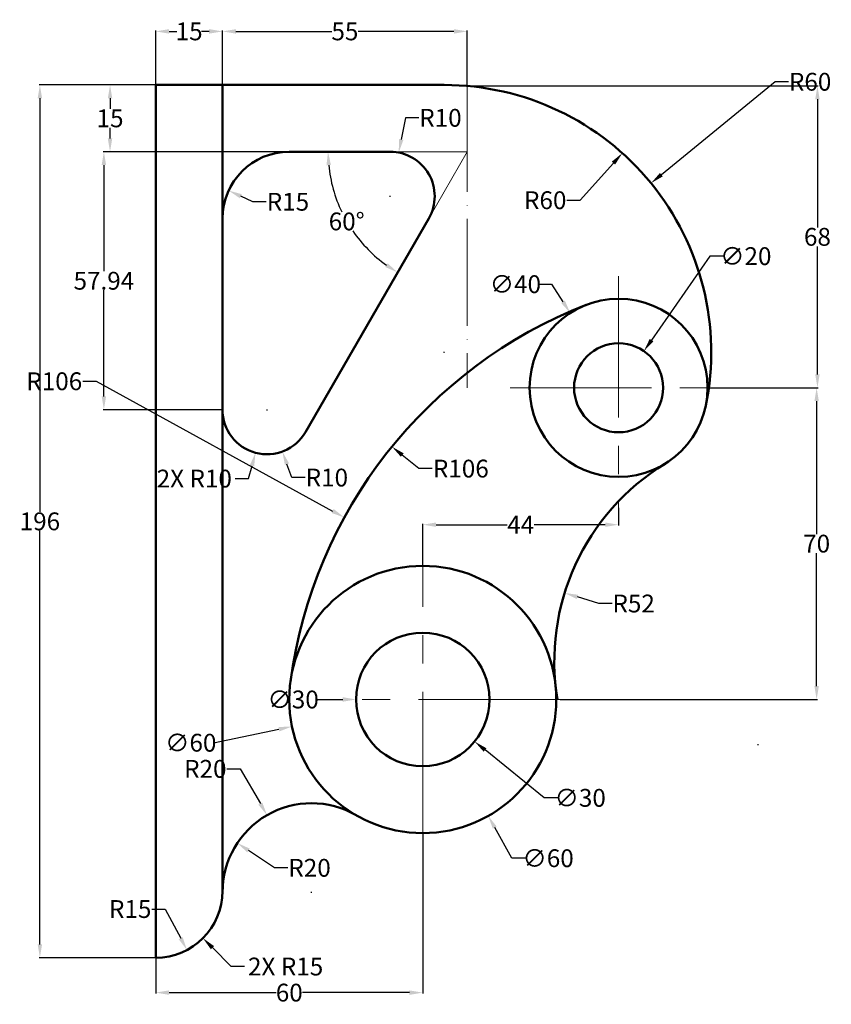
# Model space of a CAD drawing. Units: inches. Extents: x 88 to 270, y 37 to 259.
import ezdxf

# ---------------------------------------------------------------- set-up
doc = ezdxf.new("R2010")
doc.units = ezdxf.units.IN
doc.header["$MEASUREMENT"] = 0
doc.linetypes.add('ACAD_ISO04W100', pattern=[30, 24, -3, 0, -3])
doc.linetypes.add('CENTER', pattern=[50.8, 31.75, -6.35, 6.35, -6.35])
for name, color, linetype, lineweight in [('M-CNTR', 4, 'CENTER', 18), ('M-CONS', 4, 'ACAD_ISO04W100', 13), ('M-DIMS', 2, 'Continuous', 25), ('M-OUTL', 7, 'Continuous', 50)]:
    doc.layers.add(name, color=color, linetype=linetype, lineweight=lineweight)
doc.styles.get("Standard").update_dxf_attribs({"font": 'arial.ttf'})
doc.dimstyles.get("Standard").update_dxf_attribs({"dimtxt": 4, "dimasz": 3, "dimexe": 0.18, "dimexo": 0.0625, "dimgap": 0.09, "dimtad": 0, "dimtih": 1, "dimtoh": 1, "dimdec": 0, "dimzin": 0, "dimdsep": 46, "dimtxsty": 'Standard', "dimcen": 0.09, "dimclrd": 1, "dimclre": 1, "dimadec": 0, "dimazin": 0, "dimtfac": 1, "dimtdec": 0, "dimtofl": 0, "dimtmove": 0, "dimatfit": 3, "dimfxl": 1, "dimtolj": 1, "dimtzin": 0, "dimarcsym": 0})

# ---------------------------------------------------------------- blocks, each defined once
blk = doc.blocks.new('*D1')
at = {"layer": 'Defpoints', "color": 0, "transparency": 16777216}
for p in [(118.7, 62.9), (125.71, 49.64)]:
    blk.add_point(p, dxfattribs=at)
at = {"layer": 'M-DIMS', "color": 0, "lineweight": -2, "transparency": 16777216}
for p, q in [((117.85, 58.84), (120.85, 58.84)), ((120.85, 58.84), (124.3, 52.29))]:
    blk.add_line(p, q, dxfattribs=at)
at = {"layer": 'M-DIMS', "color": 0, "transparency": 16777216}
blk.add_solid([(124.75, 52.53), (123.86, 52.06), (125.71, 49.64)], dxfattribs=at)
at = {"layer": 'M-DIMS', "color": 0, "transparency": 16777216, "insert": (112.96, 58.84), "char_height": 4, "attachment_point": 5}
blk.add_mtext('\\A1;R15', dxfattribs=at)
blk = doc.blocks.new('*D2')
at = {"layer": 'Defpoints', "color": 0, "transparency": 16777216}
for p in [(92.67, 243.9), (118.7, 243.9), (118.7, 47.9)]:
    blk.add_point(p, dxfattribs=at)
at = {"layer": 'M-DIMS', "color": 0, "lineweight": -2, "transparency": 16777216}
for p, q in [((118.63, 243.9), (92.49, 243.9)), ((92.67, 240.9), (92.67, 148.04)), ((92.67, 50.9), (92.67, 143.77)), ((118.63, 47.9), (92.49, 47.9))]:
    blk.add_line(p, q, dxfattribs=at)
at = {"layer": 'M-DIMS', "color": 0, "transparency": 16777216}
for points in [[(92.17, 240.9), (93.17, 240.9), (92.67, 243.9)], [(92.17, 50.9), (93.17, 50.9), (92.67, 47.9)]]:
    blk.add_solid(points, dxfattribs=at)
at = {"layer": 'M-DIMS', "color": 0, "transparency": 16777216, "insert": (92.67, 145.9), "char_height": 4, "attachment_point": 5}
blk.add_mtext('\\A1;196', dxfattribs=at)
blk = doc.blocks.new('*D3')
at = {"layer": 'Defpoints', "color": 0, "transparency": 16777216}
for p in [(133.7, 255.93), (118.7, 243.9), (133.7, 243.9)]:
    blk.add_point(p, dxfattribs=at)
at = {"layer": 'M-DIMS', "color": 0, "lineweight": -2, "transparency": 16777216}
for p, q in [((118.7, 243.97), (118.7, 256.11)), ((121.7, 255.93), (123.42, 255.93)), ((130.7, 255.93), (128.98, 255.93)), ((133.7, 243.97), (133.7, 256.11))]:
    blk.add_line(p, q, dxfattribs=at)
at = {"layer": 'M-DIMS', "color": 0, "transparency": 16777216}
for points in [[(121.7, 256.43), (121.7, 255.43), (118.7, 255.93)], [(130.7, 256.43), (130.7, 255.43), (133.7, 255.93)]]:
    blk.add_solid(points, dxfattribs=at)
at = {"layer": 'M-DIMS', "color": 0, "transparency": 16777216, "insert": (126.2, 255.93), "char_height": 4, "attachment_point": 5}
blk.add_mtext('\\A1;15', dxfattribs=at)
blk = doc.blocks.new('*D4')
at = {"layer": 'Defpoints', "color": 0, "transparency": 16777216}
for p in [(133.7, 243.9), (108.43, 228.9), (148.7, 228.9)]:
    blk.add_point(p, dxfattribs=at)
at = {"layer": 'M-DIMS', "color": 0, "lineweight": -2, "transparency": 16777216}
for p, q in [((133.63, 243.9), (108.25, 243.9)), ((108.43, 240.9), (108.43, 238.54)), ((108.43, 231.9), (108.43, 234.27)), ((148.63, 228.9), (108.25, 228.9))]:
    blk.add_line(p, q, dxfattribs=at)
at = {"layer": 'M-DIMS', "color": 0, "transparency": 16777216}
for points in [[(107.93, 240.9), (108.93, 240.9), (108.43, 243.9)], [(107.93, 231.9), (108.93, 231.9), (108.43, 228.9)]]:
    blk.add_solid(points, dxfattribs=at)
at = {"layer": 'M-DIMS', "color": 0, "transparency": 16777216, "insert": (108.43, 236.4), "char_height": 4, "attachment_point": 5}
blk.add_mtext('\\A1;15', dxfattribs=at)
blk = doc.blocks.new('*D5')
at = {"layer": 'Defpoints', "color": 0, "transparency": 16777216}
for p in [(188.7, 255.93), (133.7, 243.9), (188.7, 243.9)]:
    blk.add_point(p, dxfattribs=at)
at = {"layer": 'M-DIMS', "color": 0, "lineweight": -2, "transparency": 16777216}
for p, q in [((133.7, 243.97), (133.7, 256.11)), ((136.7, 255.93), (158.23, 255.93)), ((185.7, 255.93), (164.17, 255.93)), ((188.7, 243.97), (188.7, 256.11))]:
    blk.add_line(p, q, dxfattribs=at)
at = {"layer": 'M-DIMS', "color": 0, "transparency": 16777216}
for points in [[(136.7, 256.43), (136.7, 255.43), (133.7, 255.93)], [(185.7, 256.43), (185.7, 255.43), (188.7, 255.93)]]:
    blk.add_solid(points, dxfattribs=at)
at = {"layer": 'M-DIMS', "color": 0, "transparency": 16777216, "insert": (161.2, 255.93), "char_height": 4, "attachment_point": 5}
blk.add_mtext('\\A1;55', dxfattribs=at)
blk = doc.blocks.new('*D6')
at = {"layer": 'Defpoints', "color": 0, "transparency": 16777216}
for p in [(148.7, 228.9), (171.38, 228.9), (159.3, 218.2), (180.04, 213.9), (152.36, 165.96)]:
    blk.add_point(p, dxfattribs=at)
at = {"layer": 'M-DIMS', "color": 0, "lineweight": -2, "transparency": 16777216}
for start, end in [(185.4964, 205.5845), (214.6218, 234.5036)]:
    blk.add_arc((188.7, 228.9), 31.28, start, end, dxfattribs=at)
at = {"layer": 'M-DIMS', "color": 0, "transparency": 16777216}
for points in [[(157.06, 225.88), (158.06, 225.93), (157.41, 228.9)], [(170.8, 203.85), (170.26, 203.01), (173.05, 201.81)]]:
    blk.add_solid(points, dxfattribs=at)
at = {"layer": 'M-DIMS', "color": 0, "transparency": 16777216, "insert": (161.6, 213.26), "char_height": 4, "attachment_point": 5}
blk.add_mtext('\\A1;60°', dxfattribs=at)
blk = doc.blocks.new('*D7')
at = {"layer": 'Defpoints', "color": 0, "transparency": 16777216}
for p in [(135.07, 220.18), (148.7, 213.9)]:
    blk.add_point(p, dxfattribs=at)
at = {"layer": 'M-DIMS', "color": 0, "lineweight": -2, "transparency": 16777216}
for p, q in [((140.52, 217.67), (137.8, 218.93)), ((143.52, 217.67), (140.52, 217.67))]:
    blk.add_line(p, q, dxfattribs=at)
at = {"layer": 'M-DIMS', "color": 0, "transparency": 16777216}
blk.add_solid([(138.01, 219.38), (137.59, 218.47), (135.07, 220.18)], dxfattribs=at)
at = {"layer": 'M-DIMS', "color": 0, "transparency": 16777216, "insert": (148.41, 217.67), "char_height": 4, "attachment_point": 5}
blk.add_mtext('\\A1;R15', dxfattribs=at)
blk = doc.blocks.new('*D8')
at = {"layer": 'Defpoints', "color": 0, "transparency": 16777216}
for p in [(173.29, 228.72), (171.38, 218.9)]:
    blk.add_point(p, dxfattribs=at)
at = {"layer": 'M-DIMS', "color": 0, "lineweight": -2, "transparency": 16777216}
for p, q in [((174.81, 236.52), (173.86, 231.66)), ((177.81, 236.52), (174.81, 236.52)), ((171.29, 218.9), (171.47, 218.9)), ((171.38, 218.81), (171.38, 218.99))]:
    blk.add_line(p, q, dxfattribs=at)
at = {"layer": 'M-DIMS', "color": 0, "transparency": 16777216}
blk.add_solid([(173.37, 231.76), (174.35, 231.57), (173.29, 228.72)], dxfattribs=at)
at = {"layer": 'M-DIMS', "color": 0, "transparency": 16777216, "insert": (182.67, 236.52), "char_height": 4, "attachment_point": 5}
blk.add_mtext('\\A1;R10', dxfattribs=at)
blk = doc.blocks.new('*D9')
at = {"layer": 'Defpoints', "color": 0, "transparency": 16777216}
for p in [(143.7, 170.96), (147.15, 161.57)]:
    blk.add_point(p, dxfattribs=at)
at = {"layer": 'M-DIMS', "color": 0, "lineweight": -2, "transparency": 16777216}
for p, q in [((143.61, 170.96), (143.79, 170.96)), ((143.7, 170.87), (143.7, 171.05)), ((149.29, 155.74), (148.18, 158.76)), ((152.29, 155.74), (149.29, 155.74))]:
    blk.add_line(p, q, dxfattribs=at)
at = {"layer": 'M-DIMS', "color": 0, "transparency": 16777216}
blk.add_solid([(148.65, 158.93), (147.71, 158.59), (147.15, 161.57)], dxfattribs=at)
at = {"layer": 'M-DIMS', "color": 0, "transparency": 16777216, "insert": (157.15, 155.74), "char_height": 4, "attachment_point": 5}
blk.add_mtext('\\A1;R10', dxfattribs=at)
blk = doc.blocks.new('*D10')
at = {"layer": 'Defpoints', "color": 0, "transparency": 16777216}
for p in [(178.7, 75.9), (118.7, 47.9), (178.7, 40.07)]:
    blk.add_point(p, dxfattribs=at)
at = {"layer": 'M-DIMS', "color": 0, "lineweight": -2, "transparency": 16777216}
for p, q in [((178.7, 75.84), (178.7, 39.89)), ((118.7, 47.84), (118.7, 39.89)), ((121.7, 40.07), (145.74, 40.07)), ((175.7, 40.07), (151.66, 40.07))]:
    blk.add_line(p, q, dxfattribs=at)
at = {"layer": 'M-DIMS', "color": 0, "transparency": 16777216}
for points in [[(121.7, 40.57), (121.7, 39.57), (118.7, 40.07)], [(175.7, 40.57), (175.7, 39.57), (178.7, 40.07)]]:
    blk.add_solid(points, dxfattribs=at)
at = {"layer": 'M-DIMS', "color": 0, "transparency": 16777216, "insert": (148.7, 40.07), "char_height": 4, "attachment_point": 5}
blk.add_mtext('\\A1;60', dxfattribs=at)
blk = doc.blocks.new('*D11')
at = {"layer": 'Defpoints', "color": 0, "transparency": 16777216}
for p in [(137.03, 73.66), (153.7, 62.6)]:
    blk.add_point(p, dxfattribs=at)
at = {"layer": 'M-DIMS', "color": 0, "lineweight": -2, "transparency": 16777216}
for p, q in [((145.4, 68.1), (139.53, 72)), ((148.4, 68.1), (145.4, 68.1))]:
    blk.add_line(p, q, dxfattribs=at)
at = {"layer": 'M-DIMS', "color": 0, "transparency": 16777216}
blk.add_solid([(139.81, 72.42), (139.25, 71.58), (137.03, 73.66)], dxfattribs=at)
at = {"layer": 'M-DIMS', "color": 0, "transparency": 16777216, "insert": (153.26, 68.1), "char_height": 4, "attachment_point": 5}
blk.add_mtext('\\A1;R20', dxfattribs=at)
blk = doc.blocks.new('*D12')
at = {"layer": 'Defpoints', "color": 0, "transparency": 16777216}
for p in [(164, 132.06), (193.4, 79.75)]:
    blk.add_point(p, dxfattribs=at)
at = {"layer": 'M-DIMS', "color": 0, "lineweight": -2, "transparency": 16777216}
for p, q in [((178.61, 105.9), (178.79, 105.9)), ((178.7, 105.81), (178.7, 105.99)), ((198.74, 70.25), (194.87, 77.14)), ((201.74, 70.25), (198.74, 70.25))]:
    blk.add_line(p, q, dxfattribs=at)
at = {"layer": 'M-DIMS', "color": 0, "transparency": 16777216}
blk.add_solid([(195.3, 77.38), (194.43, 76.89), (193.4, 79.75)], dxfattribs=at)
at = {"layer": 'M-DIMS', "color": 0, "transparency": 16777216, "insert": (206.86, 70.25), "char_height": 4, "attachment_point": 5}
blk.add_mtext('\\A1;∅60', dxfattribs=at)
blk = doc.blocks.new('*D13')
at = {"layer": 'Defpoints', "color": 0, "transparency": 16777216}
for p in [(167.05, 115.35), (190.35, 96.45)]:
    blk.add_point(p, dxfattribs=at)
at = {"layer": 'M-DIMS', "color": 0, "lineweight": -2, "transparency": 16777216}
for p, q in [((178.61, 105.9), (178.79, 105.9)), ((178.7, 105.81), (178.7, 105.99)), ((205.94, 83.81), (192.68, 94.56)), ((208.94, 83.81), (205.94, 83.81))]:
    blk.add_line(p, q, dxfattribs=at)
at = {"layer": 'M-DIMS', "color": 0, "transparency": 16777216}
blk.add_solid([(192.99, 94.95), (192.36, 94.18), (190.35, 96.45)], dxfattribs=at)
at = {"layer": 'M-DIMS', "color": 0, "transparency": 16777216, "insert": (214.07, 83.81), "char_height": 4, "attachment_point": 5}
blk.add_mtext('\\A1;∅30', dxfattribs=at)
blk = doc.blocks.new('*D14')
at = {"layer": 'Defpoints', "color": 0, "transparency": 16777216}
for p in [(246.88, 175.9), (209.49, 105.9), (267.19, 105.9)]:
    blk.add_point(p, dxfattribs=at)
at = {"layer": 'M-DIMS', "color": 0, "lineweight": -2, "transparency": 16777216}
for p, q in [((246.95, 175.9), (267.37, 175.9)), ((267.19, 172.9), (267.19, 143.04)), ((267.19, 108.9), (267.19, 138.77)), ((209.55, 105.9), (267.37, 105.9))]:
    blk.add_line(p, q, dxfattribs=at)
at = {"layer": 'M-DIMS', "color": 0, "transparency": 16777216}
for points in [[(266.69, 172.9), (267.69, 172.9), (267.19, 175.9)], [(266.69, 108.9), (267.69, 108.9), (267.19, 105.9)]]:
    blk.add_solid(points, dxfattribs=at)
at = {"layer": 'M-DIMS', "color": 0, "transparency": 16777216, "insert": (267.19, 140.9), "char_height": 4, "attachment_point": 5}
blk.add_mtext('\\A1;70', dxfattribs=at)
blk = doc.blocks.new('*D15')
at = {"layer": 'Defpoints', "color": 0, "transparency": 16777216}
for p in [(171.77, 162.67), (254.02, 95.81)]:
    blk.add_point(p, dxfattribs=at)
at = {"layer": 'M-DIMS', "color": 0, "lineweight": -2, "transparency": 16777216}
for p, q in [((177.83, 157.75), (174.1, 160.78)), ((180.83, 157.75), (177.83, 157.75))]:
    blk.add_line(p, q, dxfattribs=at)
at = {"layer": 'M-DIMS', "color": 0, "transparency": 16777216}
blk.add_solid([(174.41, 161.17), (173.78, 160.39), (171.77, 162.67)], dxfattribs=at)
at = {"layer": 'M-DIMS', "color": 0, "transparency": 16777216, "insert": (187.25, 157.75), "char_height": 4, "attachment_point": 5}
blk.add_mtext('\\A1;R106', dxfattribs=at)
blk = doc.blocks.new('*D16')
at = {"layer": 'Defpoints', "color": 0, "transparency": 16777216}
for p in [(222.7, 148.98), (222.7, 145.15), (178.7, 135.9)]:
    blk.add_point(p, dxfattribs=at)
at = {"layer": 'M-DIMS', "color": 0, "lineweight": -2, "transparency": 16777216}
for p, q in [((222.7, 148.91), (222.7, 144.97)), ((178.7, 135.97), (178.7, 145.33)), ((181.7, 145.15), (197.67, 145.15)), ((219.7, 145.15), (203.72, 145.15))]:
    blk.add_line(p, q, dxfattribs=at)
at = {"layer": 'M-DIMS', "color": 0, "transparency": 16777216}
for points in [[(181.7, 145.65), (181.7, 144.65), (178.7, 145.15)], [(219.7, 145.65), (219.7, 144.65), (222.7, 145.15)]]:
    blk.add_solid(points, dxfattribs=at)
at = {"layer": 'M-DIMS', "color": 0, "transparency": 16777216, "insert": (200.7, 145.15), "char_height": 4, "attachment_point": 5}
blk.add_mtext('\\A1;44', dxfattribs=at)
blk = doc.blocks.new('*D17')
at = {"layer": 'Defpoints', "color": 0, "transparency": 16777216}
for p in [(210.56, 129.82), (260.25, 114.47)]:
    blk.add_point(p, dxfattribs=at)
at = {"layer": 'M-DIMS', "color": 0, "lineweight": -2, "transparency": 16777216}
for p, q in [((218.23, 127.45), (213.43, 128.93)), ((221.23, 127.45), (218.23, 127.45))]:
    blk.add_line(p, q, dxfattribs=at)
at = {"layer": 'M-DIMS', "color": 0, "transparency": 16777216}
blk.add_solid([(213.58, 129.41), (213.28, 128.45), (210.56, 129.82)], dxfattribs=at)
at = {"layer": 'M-DIMS', "color": 0, "transparency": 16777216, "insert": (226.08, 127.45), "char_height": 4, "attachment_point": 5}
blk.add_mtext('\\A1;R52', dxfattribs=at)
blk = doc.blocks.new('*D18')
at = {"layer": 'Defpoints', "color": 0, "transparency": 16777216}
for p in [(223.54, 228.59), (183.51, 183.9)]:
    blk.add_point(p, dxfattribs=at)
at = {"layer": 'M-DIMS', "color": 0, "lineweight": -2, "transparency": 16777216}
for p, q in [((214.07, 218.02), (221.54, 226.36)), ((211.07, 218.02), (214.07, 218.02))]:
    blk.add_line(p, q, dxfattribs=at)
at = {"layer": 'M-DIMS', "color": 0, "transparency": 16777216}
blk.add_solid([(221.17, 226.69), (221.91, 226.02), (223.54, 228.59)], dxfattribs=at)
at = {"layer": 'M-DIMS', "color": 0, "transparency": 16777216, "insert": (206.21, 218.02), "char_height": 4, "attachment_point": 5}
blk.add_mtext('\\A1;R60', dxfattribs=at)
blk = doc.blocks.new('*D19')
at = {"layer": 'Defpoints', "color": 0, "transparency": 16777216}
for p in [(211.83, 192.69), (233.56, 159.11)]:
    blk.add_point(p, dxfattribs=at)
at = {"layer": 'M-DIMS', "color": 0, "lineweight": -2, "transparency": 16777216}
for p, q in [((204.64, 199.17), (207.64, 199.17)), ((207.64, 199.17), (210.2, 195.21)), ((222.61, 175.9), (222.79, 175.9)), ((222.7, 175.81), (222.7, 175.99))]:
    blk.add_line(p, q, dxfattribs=at)
at = {"layer": 'M-DIMS', "color": 0, "transparency": 16777216}
blk.add_solid([(210.62, 195.48), (209.78, 194.94), (211.83, 192.69)], dxfattribs=at)
at = {"layer": 'M-DIMS', "color": 0, "transparency": 16777216, "insert": (199.51, 199.17), "char_height": 4, "attachment_point": 5}
blk.add_mtext('\\A1;∅40', dxfattribs=at)
blk = doc.blocks.new('*D20')
at = {"layer": 'Defpoints', "color": 0, "transparency": 16777216}
for p in [(228.39, 184.13), (217.01, 167.68)]:
    blk.add_point(p, dxfattribs=at)
at = {"layer": 'M-DIMS', "color": 0, "lineweight": -2, "transparency": 16777216}
for p, q in [((243.16, 205.46), (230.1, 186.59)), ((246.16, 205.46), (243.16, 205.46)), ((222.61, 175.9), (222.79, 175.9)), ((222.7, 175.81), (222.7, 175.99))]:
    blk.add_line(p, q, dxfattribs=at)
at = {"layer": 'M-DIMS', "color": 0, "transparency": 16777216}
blk.add_solid([(229.69, 186.88), (230.51, 186.31), (228.39, 184.13)], dxfattribs=at)
at = {"layer": 'M-DIMS', "color": 0, "transparency": 16777216, "insert": (251.28, 205.46), "char_height": 4, "attachment_point": 5}
blk.add_mtext('\\A1;∅20', dxfattribs=at)
blk = doc.blocks.new('*D21')
at = {"layer": 'Defpoints', "color": 0, "transparency": 16777216}
for p in [(188.7, 243.68), (242.7, 175.9), (267.37, 175.9)]:
    blk.add_point(p, dxfattribs=at)
at = {"layer": 'M-DIMS', "color": 0, "lineweight": -2, "transparency": 16777216}
for p, q in [((188.76, 243.68), (267.55, 243.68)), ((267.37, 240.68), (267.37, 211.92)), ((267.37, 178.9), (267.37, 207.66)), ((242.76, 175.9), (267.55, 175.9))]:
    blk.add_line(p, q, dxfattribs=at)
at = {"layer": 'M-DIMS', "color": 0, "transparency": 16777216}
for points in [[(266.87, 240.68), (267.87, 240.68), (267.37, 243.68)], [(266.87, 178.9), (267.87, 178.9), (267.37, 175.9)]]:
    blk.add_solid(points, dxfattribs=at)
at = {"layer": 'M-DIMS', "color": 0, "transparency": 16777216, "insert": (267.37, 209.79), "char_height": 4, "attachment_point": 5}
blk.add_mtext('\\A1;68', dxfattribs=at)
blk = doc.blocks.new('*D22')
at = {"layer": 'Defpoints', "color": 0, "transparency": 16777216}
for p in [(107.05, 228.9), (148.7, 228.9), (133.7, 170.96)]:
    blk.add_point(p, dxfattribs=at)
at = {"layer": 'M-DIMS', "color": 1, "lineweight": -2, "transparency": 16777216}
for p, q in [((148.63, 228.9), (106.87, 228.9)), ((107.05, 225.9), (107.05, 202.06)), ((107.05, 173.96), (107.05, 197.8)), ((133.63, 170.96), (106.87, 170.96))]:
    blk.add_line(p, q, dxfattribs=at)
at = {"layer": 'M-DIMS', "color": 1, "transparency": 16777216}
for points in [[(106.55, 225.9), (107.55, 225.9), (107.05, 228.9)], [(106.55, 173.96), (107.55, 173.96), (107.05, 170.96)]]:
    blk.add_solid(points, dxfattribs=at)
at = {"layer": 'M-DIMS', "color": 0, "transparency": 16777216, "insert": (107.05, 199.93), "char_height": 4, "attachment_point": 5}
blk.add_mtext('\\A1;57.94', dxfattribs=at)
blk = doc.blocks.new('*D23')
at = {"layer": 'Defpoints', "color": 0, "transparency": 16777216}
for p in [(229.98, 221.85), (183.51, 183.9)]:
    blk.add_point(p, dxfattribs=at)
at = {"layer": 'M-DIMS', "color": 1, "lineweight": -2, "transparency": 16777216}
for p, q in [((257.87, 244.62), (232.3, 223.75)), ((260.87, 244.62), (257.87, 244.62)), ((183.42, 183.9), (183.6, 183.9)), ((183.51, 183.81), (183.51, 183.99))]:
    blk.add_line(p, q, dxfattribs=at)
at = {"layer": 'M-DIMS', "color": 1, "transparency": 16777216}
blk.add_solid([(231.99, 224.14), (232.62, 223.36), (229.98, 221.85)], dxfattribs=at)
at = {"layer": 'M-DIMS', "color": 0, "transparency": 16777216, "insert": (265.73, 244.62), "char_height": 4, "attachment_point": 5}
blk.add_mtext('\\A1;R60', dxfattribs=at)
blk = doc.blocks.new('*D24')
at = {"layer": 'Defpoints', "color": 0, "transparency": 16777216}
for p in [(143.7, 79.92), (153.7, 62.6)]:
    blk.add_point(p, dxfattribs=at)
at = {"layer": 'M-DIMS', "color": 1, "lineweight": -2, "transparency": 16777216}
for p, q in [((134.7, 90.32), (137.7, 90.32)), ((137.7, 90.32), (142.2, 82.52)), ((153.61, 62.6), (153.79, 62.6)), ((153.7, 62.51), (153.7, 62.69))]:
    blk.add_line(p, q, dxfattribs=at)
at = {"layer": 'M-DIMS', "color": 1, "transparency": 16777216}
blk.add_solid([(142.63, 82.77), (141.76, 82.27), (143.7, 79.92)], dxfattribs=at)
at = {"layer": 'M-DIMS', "color": 0, "transparency": 16777216, "insert": (129.84, 90.32), "char_height": 4, "attachment_point": 5}
blk.add_mtext('\\A1;R20', dxfattribs=at)
blk = doc.blocks.new('*D25')
at = {"layer": 'Defpoints', "color": 0, "transparency": 16777216}
for p in [(118.7, 62.9), (129.3, 52.3)]:
    blk.add_point(p, dxfattribs=at)
at = {"layer": 'M-DIMS', "color": 1, "lineweight": -2, "transparency": 16777216}
for p, q in [((118.61, 62.9), (118.79, 62.9)), ((118.7, 62.81), (118.7, 62.99)), ((135.67, 45.93), (131.42, 50.18)), ((138.67, 45.93), (135.67, 45.93))]:
    blk.add_line(p, q, dxfattribs=at)
at = {"layer": 'M-DIMS', "color": 1, "transparency": 16777216}
blk.add_solid([(131.78, 50.53), (131.07, 49.82), (129.3, 52.3)], dxfattribs=at)
at = {"layer": 'M-DIMS', "color": 0, "transparency": 16777216, "insert": (147.88, 45.93), "char_height": 4, "attachment_point": 5}
blk.add_mtext('\\A1;2X R15', dxfattribs=at)
blk = doc.blocks.new('*D26')
at = {"layer": 'Defpoints', "color": 0, "transparency": 16777216}
for p in [(143.7, 170.96), (141.11, 161.3)]:
    blk.add_point(p, dxfattribs=at)
at = {"layer": 'M-DIMS', "color": 1, "lineweight": -2, "transparency": 16777216}
for p, q in [((143.61, 170.96), (143.79, 170.96)), ((143.7, 170.87), (143.7, 171.05)), ((139.56, 155.51), (140.33, 158.4)), ((136.56, 155.51), (139.56, 155.51))]:
    blk.add_line(p, q, dxfattribs=at)
at = {"layer": 'M-DIMS', "color": 1, "transparency": 16777216}
blk.add_solid([(139.85, 158.53), (140.82, 158.27), (141.11, 161.3)], dxfattribs=at)
at = {"layer": 'M-DIMS', "color": 0, "transparency": 16777216, "insert": (127.36, 155.51), "char_height": 4, "attachment_point": 5}
blk.add_mtext('\\A1;2X R10', dxfattribs=at)
blk = doc.blocks.new('*D27')
at = {"layer": 'Defpoints', "color": 0, "transparency": 16777216}
for p in [(208.08, 111.98), (149.32, 99.83)]:
    blk.add_point(p, dxfattribs=at)
at = {"layer": 'M-DIMS', "color": 1, "lineweight": -2, "transparency": 16777216}
for p, q in [((178.61, 105.9), (178.79, 105.9)), ((178.7, 105.81), (178.7, 105.99)), ((131.69, 96.19), (146.38, 99.22))]:
    blk.add_line(p, q, dxfattribs=at)
at = {"layer": 'M-DIMS', "color": 1, "transparency": 16777216}
blk.add_solid([(146.28, 99.71), (146.48, 98.73), (149.32, 99.83)], dxfattribs=at)
at = {"layer": 'M-DIMS', "color": 0, "transparency": 16777216, "insert": (126.57, 96.19), "char_height": 4, "attachment_point": 5}
blk.add_mtext('\\A1;∅60', dxfattribs=at)
blk = doc.blocks.new('*D28')
at = {"layer": 'Defpoints', "color": 0, "transparency": 16777216}
for p in [(163.7, 105.9), (193.7, 105.9)]:
    blk.add_point(p, dxfattribs=at)
at = {"layer": 'M-DIMS', "color": 1, "lineweight": -2, "transparency": 16777216}
for p, q in [((154.7, 105.9), (160.7, 105.9)), ((178.61, 105.9), (178.79, 105.9)), ((178.7, 105.81), (178.7, 105.99))]:
    blk.add_line(p, q, dxfattribs=at)
at = {"layer": 'M-DIMS', "color": 1, "transparency": 16777216}
blk.add_solid([(160.7, 106.4), (160.7, 105.4), (163.7, 105.9)], dxfattribs=at)
at = {"layer": 'M-DIMS', "color": 0, "transparency": 16777216, "insert": (149.57, 105.9), "char_height": 4, "attachment_point": 5}
blk.add_mtext('\\A1;∅30', dxfattribs=at)
blk = doc.blocks.new('*D29')
at = {"layer": 'Defpoints', "color": 0, "transparency": 16777216}
for p in [(161.08, 146.78), (254.02, 95.81)]:
    blk.add_point(p, dxfattribs=at)
at = {"layer": 'M-DIMS', "color": 1, "lineweight": -2, "transparency": 16777216}
for p, q in [((102.32, 177.36), (105.32, 177.36)), ((105.32, 177.36), (158.45, 148.22)), ((253.93, 95.81), (254.11, 95.81)), ((254.02, 95.72), (254.02, 95.9))]:
    blk.add_line(p, q, dxfattribs=at)
at = {"layer": 'M-DIMS', "color": 1, "transparency": 16777216}
blk.add_solid([(158.69, 148.66), (158.21, 147.78), (161.08, 146.78)], dxfattribs=at)
at = {"layer": 'M-DIMS', "color": 0, "transparency": 16777216, "insert": (95.9, 177.36), "char_height": 4, "attachment_point": 5}
blk.add_mtext('\\A1;R106', dxfattribs=at)

msp = doc.modelspace()

# ---------------------------------------------------------------- linework, layer by layer
at = {"layer": 'M-CNTR'}
for p, q in [((222.697, 200.957), (222.697, 148.976)), ((198.327, 175.903), (246.884, 175.903)), ((178.697, 75.903), (178.697, 135.903)), ((209.492, 105.903), (160.882, 105.903))]:
    msp.add_line(p, q, dxfattribs=at)
at = {"layer": 'M-CONS'}
for p, q in [((188.697, 243.903), (188.697, 175.903)), ((171.376, 228.903), (188.697, 228.903)), ((180.037, 213.903), (188.697, 228.903))]:
    msp.add_line(p, q, dxfattribs=at)
at = {"layer": 'M-OUTL'}
for p, q in [((118.697, 47.903), (118.697, 243.903)), ((118.697, 243.903), (133.697, 243.903)), ((133.697, 243.903), (133.697, 62.903)), ((133.697, 243.903), (183.505, 243.903)), ((133.697, 243.903), (133.697, 228.903)), ((148.697, 228.903), (171.376, 228.903)), ((180.037, 213.903), (152.357, 165.961)), ((118.697, 47.903), (118.697, 47.903))]:
    msp.add_line(p, q, dxfattribs=at)
for centre, radius in [((222.697, 175.903), 20), ((222.697, 175.903), 10), ((178.697, 105.903), 30), ((178.697, 105.903), 15)]:
    msp.add_circle(centre, radius, dxfattribs=at)
for centre, radius, start, end in [((183.505, 183.903), 60, 348.46304, 90), ((148.697, 213.903), 15, 90, 180), ((171.376, 218.903), 10, 330, 90), ((254.024, 95.812), 106, 111.36255, 172.36972), ((143.697, 170.961), 10, 180, 330), ((260.248, 114.471), 52, 121.43587, 189.48365), ((153.697, 62.602), 20, 60, 180), ((118.697, 62.903), 15, 270, 0)]:
    msp.add_arc(centre, radius, start, end, dxfattribs=at)

# ---------------------------------------------------------------- dimensions: what is measured, and where the dimension line sits
at = {"layer": 'M-DIMS'}
for base, p1, p2, picture, middle in [((133.697, 255.932), (118.697, 243.903), (133.697, 243.903), '*D3', (126.197, 255.932)), ((188.697, 255.932), (133.697, 243.903), (188.697, 243.903), '*D5', (161.197, 255.932)), ((222.697, 145.146), (178.697, 135.903), (222.697, 148.976), '*D16', (200.697, 145.146))]:
    dim = msp.add_linear_dim(base=base, p1=p1, p2=p2, dimstyle='Standard', override={"dimclrd": 0, "dimclre": 0, "dimclrt": 0}, dxfattribs=at)
    dim.commit()
    dim.dimension.update_dxf_attribs({"geometry": picture, "text_midpoint": middle})
for center, mpoint, override, picture, middle in [((183.505, 183.903), (229.981, 221.851), {"dimdec": 0, "dimlfac": 1, "dimrnd": 0, "dimzin": 0, "dimdsep": 46, "dimlunit": 2}, '*D23', (265.728, 244.619)), ((171.376, 218.903), (173.29, 228.719), {"dimclrd": 0, "dimclre": 0, "dimclrt": 0}, '*D8', (182.673, 236.523)), ((183.505, 183.903), (223.544, 228.59), {"dimclrd": 0, "dimclre": 0, "dimclrt": 0}, '*D18', (206.208, 218.016)), ((148.697, 213.903), (135.074, 220.183), {"dimclrd": 0, "dimclre": 0, "dimclrt": 0}, '*D7', (148.407, 217.671)), ((254.024, 95.812), (161.082, 146.781), {"dimdec": 0, "dimlfac": 1, "dimrnd": 0, "dimzin": 0, "dimdsep": 46, "dimlunit": 2}, '*D29', (95.895, 177.362)), ((143.697, 170.961), (147.147, 161.575), {"dimclrd": 0, "dimclre": 0, "dimclrt": 0}, '*D9', (157.153, 155.741)), ((254.024, 95.812), (171.771, 162.674), {"dimclrd": 0, "dimclre": 0, "dimclrt": 0}, '*D15', (187.249, 157.751)), ((260.248, 114.471), (210.564, 129.817), {"dimclrd": 0, "dimclre": 0, "dimclrt": 0}, '*D17', (226.079, 127.449)), ((153.697, 62.602), (143.697, 79.923), {"dimdec": 0, "dimlfac": 1, "dimrnd": 0, "dimzin": 0, "dimdsep": 46, "dimlunit": 2}, '*D24', (129.835, 90.315)), ((153.697, 62.602), (137.03, 73.657), {"dimclrd": 0, "dimclre": 0, "dimclrt": 0}, '*D11', (153.265, 68.103)), ((118.697, 62.903), (125.706, 49.642), {"dimclrd": 0, "dimclre": 0, "dimclrt": 0}, '*D1', (112.962, 58.837))]:
    dim = msp.add_radius_dim(center=center, mpoint=mpoint, dimstyle='Standard', override=override, dxfattribs=at)
    dim.commit()
    dim.dimension.update_dxf_attribs({"geometry": picture, "text_midpoint": middle, "dimtype": 164})
for base, p1, p2, override, picture, middle in [((92.672, 243.903), (118.697, 47.903), (118.697, 243.903), {"dimclrd": 0, "dimclre": 0, "dimclrt": 0}, '*D2', (92.672, 145.903)), ((108.434, 228.903), (133.697, 243.903), (148.697, 228.903), {"dimclrd": 0, "dimclre": 0, "dimclrt": 0}, '*D4', (108.434, 236.403)), ((267.368, 175.903), (188.697, 243.678), (242.697, 175.903), {"dimclrd": 0, "dimclre": 0, "dimclrt": 0}, '*D21', (267.368, 209.791)), ((107.047, 228.903), (133.697, 170.961), (148.697, 228.903), {"dimdec": 2, "dimlfac": 1, "dimrnd": 0, "dimzin": 0, "dimdsep": 46, "dimlunit": 2}, '*D22', (107.047, 199.932)), ((267.188, 105.903), (246.884, 175.903), (209.492, 105.903), {"dimclrd": 0, "dimclre": 0, "dimclrt": 0}, '*D14', (267.188, 140.903))]:
    dim = msp.add_linear_dim(base=base, p1=p1, p2=p2, angle=90, dimstyle='Standard', override=override, dxfattribs=at)
    dim.commit()
    dim.dimension.update_dxf_attribs({"geometry": picture, "text_midpoint": middle})
dim = msp.add_angular_dim_2l(base=(159.299, 218.203), line1=((180.037, 213.903), (152.357, 165.961)), line2=((148.697, 228.903), (171.376, 228.903)), dimstyle='Standard', override={"dimclrd": 0, "dimclre": 0, "dimclrt": 0}, dxfattribs=at)
dim.commit()
dim.dimension.update_dxf_attribs({"geometry": '*D6', "text_midpoint": (161.603, 213.261)})
for p1, p2, override, picture, middle in [((217.005, 167.681), (228.389, 184.125), {"dimclrd": 0, "dimclre": 0, "dimclrt": 0}, '*D20', (251.281, 205.46)), ((233.564, 159.114), (211.829, 192.693), {"dimclrd": 0, "dimclre": 0, "dimclrt": 0}, '*D19', (199.514, 199.167)), ((163.998, 132.056), (193.396, 79.751), {"dimclrd": 0, "dimclre": 0, "dimclrt": 0}, '*D12', (206.86, 70.25)), ((167.047, 115.352), (190.347, 96.455), {"dimclrd": 0, "dimclre": 0, "dimclrt": 0}, '*D13', (214.065, 83.807)), ((208.076, 111.977), (149.318, 99.83), {"dimdec": 0, "dimlfac": 1, "dimrnd": 0, "dimzin": 0, "dimdsep": 46, "dimlunit": 2}, '*D27', (131.691, 96.185)), ((193.697, 105.904), (163.697, 105.903), {"dimdec": 0, "dimlfac": 1, "dimrnd": 0, "dimzin": 0, "dimdsep": 46, "dimlunit": 2}, '*D28', (154.697, 105.903))]:
    dim = msp.add_diameter_dim_2p(p1=p1, p2=p2, dimstyle='Standard', override=override, dxfattribs=at)
    dim.commit()
    dim.dimension.update_dxf_attribs({"geometry": picture, "text_midpoint": middle, "dimtype": 163})
for center, mpoint, picture, middle in [((143.697, 170.961), (141.109, 161.302), '*D26', (127.362, 155.506)), ((118.697, 62.903), (129.303, 52.297), '*D25', (147.883, 45.933))]:
    dim = msp.add_radius_dim(center=center, mpoint=mpoint, text='2X <>', dimstyle='Standard', override={"dimdec": 0, "dimlfac": 1, "dimrnd": 0, "dimzin": 0, "dimdsep": 46, "dimlunit": 2}, dxfattribs=at)
    dim.commit()
    dim.dimension.update_dxf_attribs({"geometry": picture, "text_midpoint": middle, "dimtype": 164})
dim = msp.add_linear_dim(base=(178.697, 40.07), p1=(118.697, 47.903), p2=(178.697, 75.903), dimstyle='Standard', override={"dimclrd": 0, "dimclre": 0, "dimclrt": 0}, dxfattribs=at)
dim.commit()
dim.dimension.update_dxf_attribs({"geometry": '*D10', "text_midpoint": (148.697, 40.07), "dimtype": 160})

doc.saveas('drawing.dxf')
